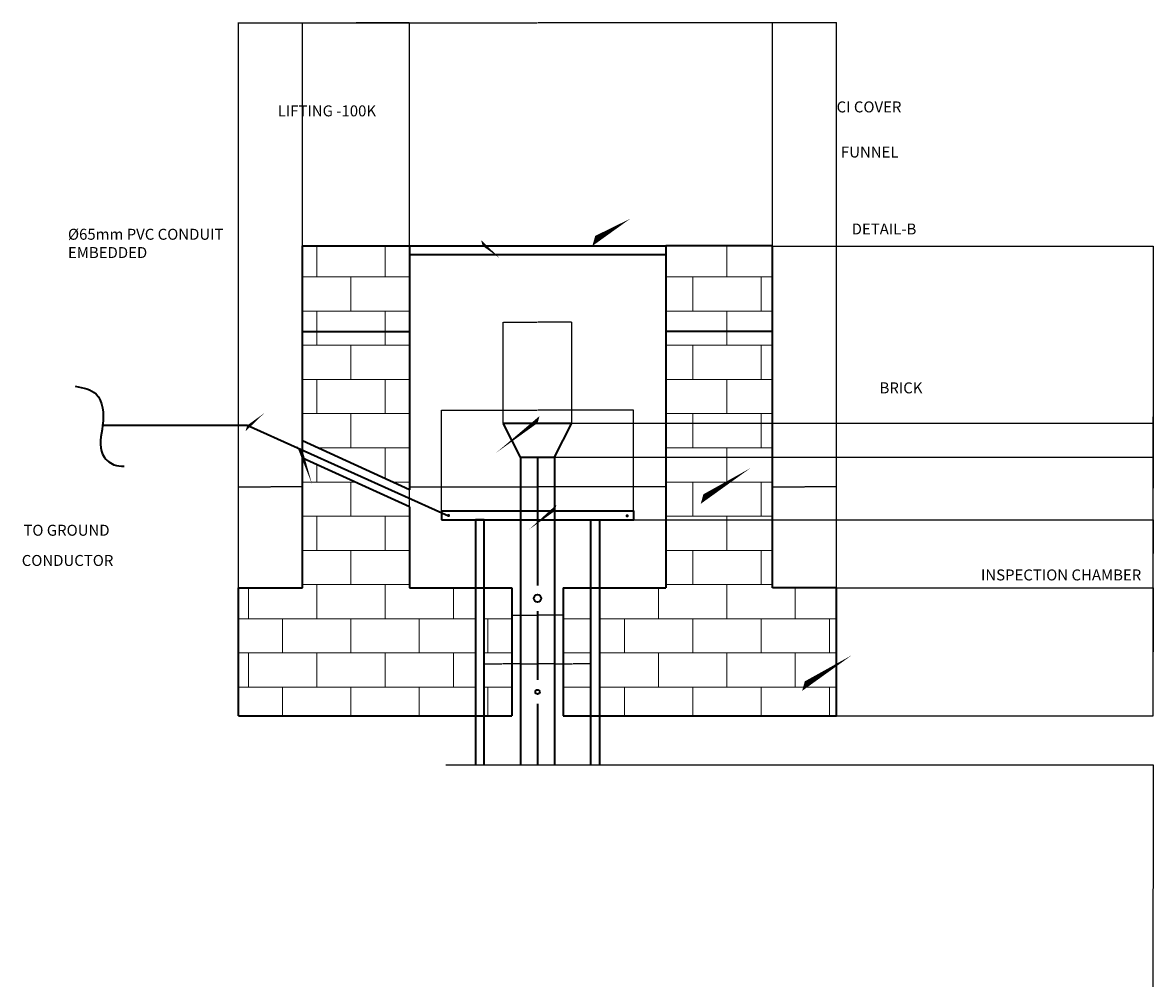
# Model space of a CAD drawing. Units: inches. Extents: x -514 to 1130, y -1450 to 978.
# Tile 2 of 2: x -224 to 1099, y -141 to 978. Entities that reach past the tile are written whole.
import ezdxf

# ---------------------------------------------------------------- set-up
doc = ezdxf.new("R2010")
doc.units = ezdxf.units.IN
doc.header["$MEASUREMENT"] = 0
for name, color, linetype, lineweight in [('A-ANNO-DIMS', 2, 'Continuous', 18), ('A-WALL', 7, 'Continuous', 35), ('A-WALL-PATT', 8, 'Continuous', 13), ('C-TOPO', 3, 'Continuous', 25), ('E-ANNO-LEAD', 2, 'Continuous', 18), ('E-ANNO-TEXT', 7, 'Continuous', 18), ('E-GRND', 1, 'Continuous', 35)]:
    doc.layers.add(name, color=color, linetype=linetype, lineweight=lineweight)
doc.styles.get("Standard").update_dxf_attribs({"font": 'arial.ttf'})
doc.dimstyles.get("Standard").update_dxf_attribs({"dimtxt": 0.18, "dimasz": 0.18, "dimexe": 0.18, "dimexo": 0.0625, "dimgap": 0.09, "dimtad": 0, "dimtih": 1, "dimtoh": 1, "dimdec": 4, "dimzin": 0, "dimdsep": 46, "dimtxsty": 'Standard', "dimcen": 0.09, "dimadec": 0, "dimazin": 0, "dimtfac": 1, "dimtdec": 4, "dimtofl": 0, "dimtmove": 0, "dimatfit": 3, "dimfxl": 1, "dimtolj": 1, "dimtzin": 0, "dimarcsym": 0})

# ---------------------------------------------------------------- blocks, each defined once
blk = doc.blocks.new('*D7')
at = {"layer": 'A-ANNO-DIMS', "color": 0, "lineweight": -2, "transparency": 16777216}
for p, q in [((103.4, 716.3), (103.4, 977.6)), ((103.6, 977.4), (378.1, 977.4)), ((653.2, 977.4), (378.7, 977.4)), ((653.4, 716.3), (653.4, 977.6))]:
    blk.add_line(p, q, dxfattribs=at)
at = {"layer": 'A-ANNO-DIMS', "color": 0, "transparency": 16777216}
for points in [[(103.6, 977.5), (103.6, 977.4), (103.4, 977.4)], [(653.2, 977.5), (653.2, 977.4), (653.4, 977.4)]]:
    blk.add_solid(points, dxfattribs=at)
at = {"layer": 'Defpoints', "color": 0, "transparency": 16777216}
for p in [(653.4, 977.4), (103.4, 716.2), (653.4, 716.2)]:
    blk.add_point(p, dxfattribs=at)
at = {"layer": 'A-ANNO-DIMS', "color": 0, "transparency": 16777216, "insert": (378.4, 977.4), "char_height": 0.18, "attachment_point": 5}
blk.add_mtext('\\A1;550', dxfattribs=at)
blk = doc.blocks.new('*D8')
at = {"layer": 'A-ANNO-DIMS', "color": 0, "lineweight": -2, "transparency": 16777216}
for p, q in [((103.4, 716.3), (103.4, 977.6)), ((103.6, 977.4), (165.6, 977.4)), ((228.2, 977.4), (166.2, 977.4)), ((228.4, 716.3), (228.4, 977.6))]:
    blk.add_line(p, q, dxfattribs=at)
at = {"layer": 'A-ANNO-DIMS', "color": 0, "transparency": 16777216}
for points in [[(103.6, 977.5), (103.6, 977.4), (103.4, 977.4)], [(228.2, 977.5), (228.2, 977.4), (228.4, 977.4)]]:
    blk.add_solid(points, dxfattribs=at)
at = {"layer": 'Defpoints', "color": 0, "transparency": 16777216}
for p in [(228.4, 977.4), (103.4, 716.2), (228.4, 716.2)]:
    blk.add_point(p, dxfattribs=at)
at = {"layer": 'A-ANNO-DIMS', "color": 0, "transparency": 16777216, "insert": (165.9, 977.4), "char_height": 0.18, "attachment_point": 5}
blk.add_mtext('\\A1;125', dxfattribs=at)
blk = doc.blocks.new('*D9')
at = {"layer": 'A-ANNO-DIMS', "color": 0, "lineweight": -2, "transparency": 16777216}
for p, q in [((228.4, 316.3), (228.4, 434.4)), ((228.6, 434.2), (378.1, 434.2)), ((528.2, 434.2), (378.7, 434.2)), ((528.4, 316.3), (528.4, 434.4))]:
    blk.add_line(p, q, dxfattribs=at)
at = {"layer": 'A-ANNO-DIMS', "color": 0, "transparency": 16777216}
for points in [[(228.6, 434.3), (228.6, 434.2), (228.4, 434.2)], [(528.2, 434.3), (528.2, 434.2), (528.4, 434.2)]]:
    blk.add_solid(points, dxfattribs=at)
at = {"layer": 'Defpoints', "color": 0, "transparency": 16777216}
for p in [(528.4, 434.2), (228.4, 316.2), (528.4, 316.2)]:
    blk.add_point(p, dxfattribs=at)
at = {"layer": 'A-ANNO-DIMS', "color": 0, "transparency": 16777216, "insert": (378.4, 434.2), "char_height": 0.18, "attachment_point": 5}
blk.add_mtext('\\A1;300', dxfattribs=at)
blk = doc.blocks.new('*D10')
at = {"layer": 'A-ANNO-DIMS', "color": 0, "lineweight": -2, "transparency": 16777216}
for p, q in [((28.4, 316.3), (28.4, 977.6)), ((28.6, 977.4), (378.1, 977.4)), ((728.2, 977.4), (378.7, 977.4)), ((728.4, 316.3), (728.4, 977.6))]:
    blk.add_line(p, q, dxfattribs=at)
at = {"layer": 'A-ANNO-DIMS', "color": 0, "transparency": 16777216}
for points in [[(28.6, 977.5), (28.6, 977.4), (28.4, 977.4)], [(728.2, 977.5), (728.2, 977.4), (728.4, 977.4)]]:
    blk.add_solid(points, dxfattribs=at)
at = {"layer": 'Defpoints', "color": 0, "transparency": 16777216}
for p in [(728.4, 977.4), (28.4, 316.2), (728.4, 316.2)]:
    blk.add_point(p, dxfattribs=at)
at = {"layer": 'A-ANNO-DIMS', "color": 0, "transparency": 16777216, "insert": (378.4, 977.4), "char_height": 0.18, "attachment_point": 5}
blk.add_mtext('\\A1;700', dxfattribs=at)
blk = doc.blocks.new('*D11')
at = {"layer": 'A-ANNO-DIMS', "color": 0, "lineweight": -2, "transparency": 16777216}
for p, q in [((28.4, 316.3), (28.4, 434.4)), ((28.6, 434.2), (65.7, 434.2)), ((103.2, 434.2), (66.1, 434.2)), ((103.4, 316.3), (103.4, 434.4))]:
    blk.add_line(p, q, dxfattribs=at)
at = {"layer": 'A-ANNO-DIMS', "color": 0, "transparency": 16777216}
for points in [[(28.6, 434.3), (28.6, 434.2), (28.4, 434.2)], [(103.2, 434.3), (103.2, 434.2), (103.4, 434.2)]]:
    blk.add_solid(points, dxfattribs=at)
at = {"layer": 'Defpoints', "color": 0, "transparency": 16777216}
for p in [(103.4, 434.2), (28.4, 316.2), (103.4, 316.2)]:
    blk.add_point(p, dxfattribs=at)
at = {"layer": 'A-ANNO-DIMS', "color": 0, "transparency": 16777216, "insert": (65.9, 434.2), "char_height": 0.18, "attachment_point": 5}
blk.add_mtext('\\A1;75', dxfattribs=at)
blk = doc.blocks.new('*D12')
at = {"layer": 'A-ANNO-DIMS', "color": 0, "lineweight": -2, "transparency": 16777216}
for p, q in [((653.4, 316.3), (653.4, 434.4)), ((653.6, 434.2), (690.7, 434.2)), ((728.2, 434.2), (691.1, 434.2)), ((728.4, 316.3), (728.4, 434.4))]:
    blk.add_line(p, q, dxfattribs=at)
at = {"layer": 'A-ANNO-DIMS', "color": 0, "transparency": 16777216}
for points in [[(653.6, 434.3), (653.6, 434.2), (653.4, 434.2)], [(728.2, 434.3), (728.2, 434.2), (728.4, 434.2)]]:
    blk.add_solid(points, dxfattribs=at)
at = {"layer": 'Defpoints', "color": 0, "transparency": 16777216}
for p in [(728.4, 434.2), (653.4, 316.2), (728.4, 316.2)]:
    blk.add_point(p, dxfattribs=at)
at = {"layer": 'A-ANNO-DIMS', "color": 0, "transparency": 16777216, "insert": (690.9, 434.2), "char_height": 0.18, "attachment_point": 5}
blk.add_mtext('\\A1;75', dxfattribs=at)
blk = doc.blocks.new('*D13')
at = {"layer": 'A-ANNO-DIMS', "color": 0, "lineweight": -2, "transparency": 16777216}
for p, q in [((348.4, 166.3), (348.4, 284.4)), ((348.6, 284.2), (378.2, 284.2)), ((408.2, 284.2), (378.6, 284.2)), ((408.4, 166.3), (408.4, 284.4))]:
    blk.add_line(p, q, dxfattribs=at)
at = {"layer": 'A-ANNO-DIMS', "color": 0, "transparency": 16777216}
for points in [[(348.6, 284.3), (348.6, 284.2), (348.4, 284.2)], [(408.2, 284.3), (408.2, 284.2), (408.4, 284.2)]]:
    blk.add_solid(points, dxfattribs=at)
at = {"layer": 'Defpoints', "color": 0, "transparency": 16777216}
for p in [(408.4, 284.2), (348.4, 166.2), (408.4, 166.2)]:
    blk.add_point(p, dxfattribs=at)
at = {"layer": 'A-ANNO-DIMS', "color": 0, "transparency": 16777216, "insert": (378.4, 284.2), "char_height": 0.18, "attachment_point": 5}
blk.add_mtext('\\A1;60', dxfattribs=at)
blk = doc.blocks.new('*D14')
at = {"layer": 'A-ANNO-DIMS', "color": 0, "lineweight": -2, "transparency": 16777216}
for p, q in [((653.5, 716.2), (1099, 716.2)), ((1098.9, 716.1), (1098.9, 516.4)), ((1098.9, 316.4), (1098.9, 516.1)), ((653.5, 316.2), (1099, 316.2))]:
    blk.add_line(p, q, dxfattribs=at)
at = {"layer": 'A-ANNO-DIMS', "color": 0, "transparency": 16777216}
for points in [[(1098.8, 716.1), (1098.9, 716.1), (1098.9, 716.2)], [(1098.8, 316.4), (1098.9, 316.4), (1098.9, 316.2)]]:
    blk.add_solid(points, dxfattribs=at)
at = {"layer": 'Defpoints', "color": 0, "transparency": 16777216}
for p in [(653.4, 716.2), (1098.9, 716.2), (653.4, 316.2)]:
    blk.add_point(p, dxfattribs=at)
at = {"layer": 'A-ANNO-DIMS', "color": 0, "transparency": 16777216, "insert": (1098.9, 516.2), "char_height": 0.18, "attachment_point": 5}
blk.add_mtext('\\A1;400', dxfattribs=at)
blk = doc.blocks.new('*D15')
at = {"layer": 'A-ANNO-DIMS', "color": 0, "lineweight": -2, "transparency": 16777216}
for p, q in [((728.5, 316.2), (1099, 316.2)), ((1098.9, 316.1), (1098.9, 241.4)), ((1098.9, 166.4), (1098.9, 241.1)), ((728.5, 166.2), (1099, 166.2))]:
    blk.add_line(p, q, dxfattribs=at)
at = {"layer": 'A-ANNO-DIMS', "color": 0, "transparency": 16777216}
for points in [[(1098.8, 316.1), (1098.9, 316.1), (1098.9, 316.2)], [(1098.8, 166.4), (1098.9, 166.4), (1098.9, 166.2)]]:
    blk.add_solid(points, dxfattribs=at)
at = {"layer": 'Defpoints', "color": 0, "transparency": 16777216}
for p in [(728.4, 316.2), (1098.9, 316.2), (728.4, 166.2)]:
    blk.add_point(p, dxfattribs=at)
at = {"layer": 'A-ANNO-DIMS', "color": 0, "transparency": 16777216, "insert": (1098.9, 241.2), "char_height": 0.18, "attachment_point": 5}
blk.add_mtext('\\A1;150', dxfattribs=at)
blk = doc.blocks.new('*D16')
at = {"layer": 'A-ANNO-DIMS', "color": 0, "lineweight": -2, "transparency": 16777216}
for p, q in [((653.5, 716.2), (1099, 716.2)), ((1098.9, 716.1), (1098.9, 441.4)), ((1098.9, 166.4), (1098.9, 441.1)), ((728.5, 166.2), (1099, 166.2))]:
    blk.add_line(p, q, dxfattribs=at)
at = {"layer": 'A-ANNO-DIMS', "color": 0, "transparency": 16777216}
for points in [[(1098.8, 716.1), (1098.9, 716.1), (1098.9, 716.2)], [(1098.8, 166.4), (1098.9, 166.4), (1098.9, 166.2)]]:
    blk.add_solid(points, dxfattribs=at)
at = {"layer": 'Defpoints', "color": 0, "transparency": 16777216}
for p in [(653.4, 716.2), (1098.9, 716.2), (728.4, 166.2)]:
    blk.add_point(p, dxfattribs=at)
at = {"layer": 'A-ANNO-DIMS', "color": 0, "transparency": 16777216, "insert": (1098.9, 441.2), "char_height": 0.18, "attachment_point": 5}
blk.add_mtext('\\A1;550', dxfattribs=at)
blk = doc.blocks.new('*D17')
at = {"layer": 'A-ANNO-DIMS', "color": 0, "lineweight": -2, "transparency": 16777216}
for p, q in [((338.3, 509.1), (338.3, 627.2)), ((338.5, 627), (378, 627)), ((418.3, 627), (378.8, 627)), ((418.5, 509.1), (418.5, 627.2))]:
    blk.add_line(p, q, dxfattribs=at)
at = {"layer": 'A-ANNO-DIMS', "color": 0, "transparency": 16777216}
for points in [[(338.5, 627), (338.5, 627), (338.3, 627)], [(418.3, 627), (418.3, 627), (418.5, 627)]]:
    blk.add_solid(points, dxfattribs=at)
at = {"layer": 'Defpoints', "color": 0, "transparency": 16777216}
for p in [(418.5, 627), (338.3, 509), (418.5, 509)]:
    blk.add_point(p, dxfattribs=at)
at = {"layer": 'A-ANNO-DIMS', "color": 0, "transparency": 16777216, "insert": (378.4, 627), "char_height": 0.18, "attachment_point": 5}
blk.add_mtext('\\A1;80.24', dxfattribs=at)
blk = doc.blocks.new('*D18')
at = {"layer": 'A-ANNO-DIMS', "color": 0, "lineweight": -2, "transparency": 16777216}
for p, q in [((265.9, 406), (265.9, 524.1)), ((266.1, 523.9), (378.1, 523.9)), ((490.7, 523.9), (378.7, 523.9)), ((490.9, 406), (490.9, 524.1))]:
    blk.add_line(p, q, dxfattribs=at)
at = {"layer": 'A-ANNO-DIMS', "color": 0, "transparency": 16777216}
for points in [[(266.1, 524), (266.1, 523.9), (265.9, 523.9)], [(490.7, 524), (490.7, 523.9), (490.9, 523.9)]]:
    blk.add_solid(points, dxfattribs=at)
at = {"layer": 'Defpoints', "color": 0, "transparency": 16777216}
for p in [(490.9, 523.9), (265.9, 405.9), (490.9, 405.9)]:
    blk.add_point(p, dxfattribs=at)
at = {"layer": 'A-ANNO-DIMS', "color": 0, "transparency": 16777216, "insert": (378.4, 523.9), "char_height": 0.18, "attachment_point": 5}
blk.add_mtext('\\A1;225', dxfattribs=at)
blk = doc.blocks.new('*D19')
at = {"layer": 'A-ANNO-DIMS', "color": 0, "lineweight": -2, "transparency": 16777216}
for p, q in [((491, 395.9), (1099, 395.9)), ((1098.9, 395.8), (1098.9, 356.3)), ((1098.9, 316.4), (1098.9, 355.9)), ((728.5, 316.2), (1099, 316.2))]:
    blk.add_line(p, q, dxfattribs=at)
at = {"layer": 'A-ANNO-DIMS', "color": 0, "transparency": 16777216}
for points in [[(1098.8, 395.8), (1098.9, 395.8), (1098.9, 395.9)], [(1098.8, 316.4), (1098.9, 316.4), (1098.9, 316.2)]]:
    blk.add_solid(points, dxfattribs=at)
at = {"layer": 'Defpoints', "color": 0, "transparency": 16777216}
for p in [(490.9, 395.9), (1098.9, 395.9), (728.4, 316.2)]:
    blk.add_point(p, dxfattribs=at)
at = {"layer": 'A-ANNO-DIMS', "color": 0, "transparency": 16777216, "insert": (1098.9, 356.1), "char_height": 0.18, "attachment_point": 5}
blk.add_mtext('\\A1;79.7', dxfattribs=at)
blk = doc.blocks.new('*D20')
at = {"layer": 'A-ANNO-DIMS', "color": 0, "lineweight": -2, "transparency": 16777216}
for p, q in [((398.5, 469), (1099, 469)), ((1098.9, 468.8), (1098.9, 432.7)), ((1098.9, 396.1), (1098.9, 432.3)), ((491, 395.9), (1099, 395.9))]:
    blk.add_line(p, q, dxfattribs=at)
at = {"layer": 'A-ANNO-DIMS', "color": 0, "transparency": 16777216}
for points in [[(1098.8, 468.8), (1098.9, 468.8), (1098.9, 469)], [(1098.8, 396.1), (1098.9, 396.1), (1098.9, 395.9)]]:
    blk.add_solid(points, dxfattribs=at)
at = {"layer": 'Defpoints', "color": 0, "transparency": 16777216}
for p in [(398.4, 469), (1098.9, 469), (490.9, 395.9)]:
    blk.add_point(p, dxfattribs=at)
at = {"layer": 'A-ANNO-DIMS', "color": 0, "transparency": 16777216, "insert": (1098.9, 432.5), "char_height": 0.18, "attachment_point": 5}
blk.add_mtext('\\A1;73.06', dxfattribs=at)
blk = doc.blocks.new('*D21')
at = {"layer": 'A-ANNO-DIMS', "color": 0, "lineweight": -2, "transparency": 16777216}
for p, q in [((418.6, 509), (1099, 509)), ((1098.9, 508.8), (1098.9, 489.2)), ((1098.9, 469.2), (1098.9, 488.8)), ((398.5, 469), (1099, 469))]:
    blk.add_line(p, q, dxfattribs=at)
at = {"layer": 'A-ANNO-DIMS', "color": 0, "transparency": 16777216}
for points in [[(1098.8, 508.8), (1098.9, 508.8), (1098.9, 509)], [(1098.8, 469.2), (1098.9, 469.2), (1098.9, 469)]]:
    blk.add_solid(points, dxfattribs=at)
at = {"layer": 'Defpoints', "color": 0, "transparency": 16777216}
for p in [(418.5, 509), (1098.9, 509), (398.4, 469)]:
    blk.add_point(p, dxfattribs=at)
at = {"layer": 'A-ANNO-DIMS', "color": 0, "transparency": 16777216, "insert": (1098.9, 489), "char_height": 0.18, "attachment_point": 5}
blk.add_mtext('\\A1;40', dxfattribs=at)
blk = doc.blocks.new('*D22')
at = {"layer": 'A-ANNO-DIMS', "color": 0, "lineweight": -2, "transparency": 16777216}
for p, q in [((491.3, 109.1), (1099, 109.1)), ((1098.9, 108.9), (1098.9, -35.7)), ((1098.9, -180.7), (1098.9, -36.1)), ((491.3, -180.9), (1099, -180.9))]:
    blk.add_line(p, q, dxfattribs=at)
at = {"layer": 'A-ANNO-DIMS', "color": 0, "transparency": 16777216}
for points in [[(1098.8, 108.9), (1098.9, 108.9), (1098.9, 109.1)], [(1098.8, -180.7), (1098.9, -180.7), (1098.9, -180.9)]]:
    blk.add_solid(points, dxfattribs=at)
at = {"layer": 'Defpoints', "color": 0, "transparency": 16777216}
for p in [(491.2, 109.1), (491.2, -180.9), (1098.9, -180.9)]:
    blk.add_point(p, dxfattribs=at)
at = {"layer": 'A-ANNO-DIMS', "color": 0, "transparency": 16777216, "insert": (1098.9, -35.9), "char_height": 0.18, "attachment_point": 5}
blk.add_mtext('\\A1;290', dxfattribs=at)
blk = doc.blocks.new('*D23')
at = {"layer": 'A-ANNO-DIMS', "color": 0, "lineweight": -2, "transparency": 16777216}
for p, q in [((315.9, 109.2), (315.9, 227.3)), ((316.1, 227.1), (336.8, 227.1)), ((358.2, 227.1), (337.5, 227.1)), ((358.4, 109.2), (358.4, 227.3))]:
    blk.add_line(p, q, dxfattribs=at)
at = {"layer": 'A-ANNO-DIMS', "color": 0, "transparency": 16777216}
for points in [[(316.1, 227.1), (316.1, 227.1), (315.9, 227.1)], [(358.2, 227.1), (358.2, 227.1), (358.4, 227.1)]]:
    blk.add_solid(points, dxfattribs=at)
at = {"layer": 'Defpoints', "color": 0, "transparency": 16777216}
for p in [(358.4, 227.1), (315.9, 109.1), (358.4, 109.1)]:
    blk.add_point(p, dxfattribs=at)
at = {"layer": 'A-ANNO-DIMS', "color": 0, "transparency": 16777216, "insert": (337.2, 227.1), "char_height": 0.18, "attachment_point": 5}
blk.add_mtext('\\A1;42.5', dxfattribs=at)
blk = doc.blocks.new('*D24')
at = {"layer": 'A-ANNO-DIMS', "color": 0, "lineweight": -2, "transparency": 16777216}
for p, q in [((358.4, 109.2), (358.4, 227.3)), ((358.6, 227.1), (378.2, 227.1)), ((398.2, 227.1), (378.6, 227.1)), ((398.4, 109.2), (398.4, 227.3))]:
    blk.add_line(p, q, dxfattribs=at)
at = {"layer": 'A-ANNO-DIMS', "color": 0, "transparency": 16777216}
for points in [[(358.6, 227.1), (358.6, 227.1), (358.4, 227.1)], [(398.2, 227.1), (398.2, 227.1), (398.4, 227.1)]]:
    blk.add_solid(points, dxfattribs=at)
at = {"layer": 'Defpoints', "color": 0, "transparency": 16777216}
for p in [(398.4, 227.1), (358.4, 109.1), (398.4, 109.1)]:
    blk.add_point(p, dxfattribs=at)
at = {"layer": 'A-ANNO-DIMS', "color": 0, "transparency": 16777216, "insert": (378.4, 227.1), "char_height": 0.18, "attachment_point": 5}
blk.add_mtext('\\A1;40', dxfattribs=at)
blk = doc.blocks.new('*D25')
at = {"layer": 'A-ANNO-DIMS', "color": 0, "lineweight": -2, "transparency": 16777216}
for p, q in [((398.4, 109.2), (398.4, 227.3)), ((398.6, 227.1), (419.3, 227.1)), ((440.7, 227.1), (420, 227.1)), ((440.9, 109.2), (440.9, 227.3))]:
    blk.add_line(p, q, dxfattribs=at)
at = {"layer": 'A-ANNO-DIMS', "color": 0, "transparency": 16777216}
for points in [[(398.6, 227.1), (398.6, 227.1), (398.4, 227.1)], [(440.7, 227.1), (440.7, 227.1), (440.9, 227.1)]]:
    blk.add_solid(points, dxfattribs=at)
at = {"layer": 'Defpoints', "color": 0, "transparency": 16777216}
for p in [(440.9, 227.1), (398.4, 109.1), (440.9, 109.1)]:
    blk.add_point(p, dxfattribs=at)
at = {"layer": 'A-ANNO-DIMS', "color": 0, "transparency": 16777216, "insert": (419.7, 227.1), "char_height": 0.18, "attachment_point": 5}
blk.add_mtext('\\A1;42.5', dxfattribs=at)

msp = doc.modelspace()

# ---------------------------------------------------------------- hatches: boundary and pattern name
at = {"layer": 'A-WALL-PATT'}
h = msp.add_hatch(dxfattribs=at)
h.set_pattern_fill('AR-B816', color=256, scale=5)
h.paths.add_polyline_path([(653.4114, 616.249), (528.4114, 616.249), (528.4114, 316.249), (450.9114, 316.249), (450.9114, 166.249), (728.4114, 166.249), (728.4114, 316.249), (653.4114, 316.249)])
h.paths.add_polyline_path([(305.9114, 316.249), (228.4114, 316.249), (228.4114, 410.9574), (103.4114, 468.1138), (103.4114, 316.249), (28.4114, 316.249), (28.4114, 166.249), (305.9114, 166.249)])
h.paths.add_polyline_path([(228.4114, 616.249), (103.4114, 616.249), (103.4114, 488.1138), (228.4114, 430.9574)])
h.paths.add_polyline_path([(228.4114, 716.249), (103.4114, 716.249), (103.4114, 616.249), (228.4114, 616.249)])
h.paths.add_polyline_path([(653.4114, 716.249), (528.4114, 716.249), (528.4114, 616.249), (653.4114, 616.249)])
h.paths.add_polyline_path([(440.9114, 316.249), (408.4114, 316.249), (408.4114, 166.249), (440.9114, 166.249)])
h.paths.add_polyline_path([(348.4114, 316.249), (315.9114, 316.249), (315.9114, 166.249), (348.4114, 166.249)])

# ---------------------------------------------------------------- linework, layer by layer
at = {"layer": 'A-WALL'}
for p, q in [((103.4114, 616.249), (103.4114, 716.249)), ((103.4114, 716.249), (228.4114, 716.249)), ((228.4114, 716.249), (228.4114, 430.9574)), ((228.4114, 716.249), (528.4114, 716.249)), ((653.4114, 716.249), (528.4114, 716.249)), ((528.4114, 716.249), (528.4114, 316.249)), ((653.4114, 616.249), (653.4114, 716.249)), ((228.4114, 706.249), (528.4114, 706.249)), ((103.4114, 316.249), (103.4114, 616.249)), ((103.4114, 616.249), (228.4114, 616.249)), ((653.4114, 616.249), (528.4114, 616.249)), ((653.4114, 316.249), (653.4114, 616.249)), ((228.4114, 410.9574), (228.4114, 316.249)), ((28.4114, 166.249), (28.4114, 316.249)), ((28.4114, 316.249), (103.4114, 316.249)), ((228.4114, 316.249), (348.4114, 316.249)), ((348.4114, 316.249), (348.4114, 166.249)), ((408.4114, 316.249), (408.4114, 166.249)), ((408.4114, 316.249), (528.4114, 316.249)), ((728.4114, 316.249), (653.4114, 316.249)), ((728.4114, 166.249), (728.4114, 316.249)), ((28.4114, 166.249), (348.4114, 166.249)), ((408.4114, 166.249), (728.4114, 166.249))]:
    msp.add_line(p, q, dxfattribs=at)
at = {"layer": 'C-TOPO'}
msp.add_line((270.9153, 109.1003), (491.2068, 109.1003), dxfattribs=at)
at = {"layer": 'E-ANNO-LEAD'}
for points in [[(314.2552, 716.249, 0, 13.2101, 0), (303.4419, 731.6936, 0, 0, 0), (176.2337, 854.7943, 0, 0, 0), (78.7042, 854.7943, 0, 0, 0)], [(442.5675, 716.249, 0, 13.2101, 0), (453.3808, 731.6936, 0, 0, 0), (713.8075, 859.4291, 0, 0, 0), (811.337, 859.4291, 0, 0, 0)], [(378.4114, 509.005, 0, 13.2101, 0), (389.2247, 524.4496, 0, 0, 0), (720.5228, 805.2712, 0, 0, 0), (818.0523, 805.2712, 0, 0, 0)], [(103.4114, 477.0187, 0, 13.2101, 0), (92.5981, 492.4634, 0, 0, 0), (5.3322, 711.6798, 0, 0, 0), (-92.1973, 711.6798, 0, 0, 0)], [(398.4114, 405.9479, 0, 13.2101, 0), (409.2247, 421.3926, 0, 0, 0), (733.0904, 715.2065, 0, 0, 0), (830.6199, 715.2065, 0, 0, 0)], [(569.3742, 414.4714, 0, 13.2101, 0), (580.1875, 429.9161, 0, 0, 0), (764.6621, 532.5402, 0, 0, 0), (862.1916, 532.5402, 0, 0, 0)], [(38.6026, 506.271, 0, 13.2101, 0), (27.7893, 490.8264, 0, 0, 0), (-99.419, 367.7257, 0, 0, 0), (-196.9485, 367.7257, 0, 0, 0)], [(688.0417, 195.5595, 0, 13.2101, 0), (698.8551, 211.0042, 0, 0, 0), (883.3297, 313.6283, 0, 0, 0), (980.8592, 313.6283, 0, 0, 0)]]:
    msp.add_lwpolyline(points, format="xyseb", dxfattribs=at)
at = {"layer": 'E-GRND'}
for p, q in [((338.2929, 509.005), (418.5299, 509.005)), ((358.4114, 469.005), (338.2929, 509.005)), ((398.4114, 469.005), (418.5299, 509.005)), ((228.4114, 430.9574), (103.4114, 488.1138)), ((228.4114, 410.9574), (103.4114, 468.1138)), ((358.4114, 469.005), (358.4114, 109.1003)), ((358.4114, 469.005), (398.4114, 469.005)), ((378.4114, 469.005), (378.4114, 318.8462)), ((398.4114, 469.005), (398.4114, 109.1003)), ((378.4114, 289.0527), (378.4114, 208.3643)), ((378.4114, 180.477), (378.4114, 109.1003))]:
    msp.add_line(p, q, dxfattribs=at)
for points in [[(274.1943, 399.9336), (38.6026, 506.271), (-130.6439, 506.271)], [(315.9114, 109.1003), (315.9114, 395.9479), (305.9114, 395.9479), (305.9114, 109.1003)], [(440.9114, 109.1003), (440.9114, 395.9479), (450.9114, 395.9479), (450.9114, 109.1003)]]:
    msp.add_lwpolyline(points, dxfattribs=at)
msp.add_lwpolyline([(265.9114, 395.9479), (490.9114, 395.9479), (490.9114, 405.9479), (265.9114, 405.9479)], close=True, dxfattribs=at)
at = {"layer": 'E-GRND', "const_width": 1.8371}
for points in [[(273.2757, 400.8522, 1), (275.1129, 400.8522, 1)], [(482.4261, 400.4516, 1), (484.2632, 400.4516, 1)]]:
    msp.add_lwpolyline(points, format="xyb", close=True, dxfattribs=at)
at = {"layer": 'E-GRND'}
for centre, radius in [((378.4114, 303.8804), 4.3406), ((378.4114, 194.3618), 2.5732)]:
    msp.add_circle(centre, radius, dxfattribs=at)
msp.add_open_spline([(-162.6127, 552.2927), (-153.2664, 550.3376), (-130.5747, 545.5911), (-128.2521, 506.4742), (-137.3734, 476.2741), (-119.6812, 459.0706), (-109.4357, 458.5737), (-105.257, 458.371)], degree=3, knots=[0, 0, 0, 0, 26.188829756, 63.58266363, 97.394470601, 115.34887117, 127.715725173, 127.715725173, 127.715725173, 127.715725173], dxfattribs=at)

# ---------------------------------------------------------------- texts
at = {"layer": 'E-ANNO-TEXT'}
for s, height, p in [('LIFTING -100K', 12.829888, (74.311, 867.9068)), ('CI COVER', 12.82989, (728.424, 872.5415)), ('FUNNEL', 12.82989, (733.4808, 819.7636)), ('DETAIL-B', 12.82989, (746.0484, 729.6989)), ('BRICK', 12.82989, (778.6886, 543.775)), ('TO GROUND', 12.82989, (-223.3294, 377.1509)), ('CONDUCTOR', 12.82989, (-225.2744, 341.7834)), ('INSPECTION CHAMBER', 12.829888, (897.3561, 324.863))]:
    msp.add_text(s, height=height, dxfattribs=at).set_placement(p)
at = {"layer": 'E-ANNO-TEXT', "insert": (-171.1715, 736.3474), "char_height": 12.829888, "width": 218.032909, "attachment_point": 1}
msp.add_mtext('%%C65mm PVC CONDUIT\\PEMBEDDED', dxfattribs=at)

# ---------------------------------------------------------------- dimensions: what is measured, and where the dimension line sits
at = {"layer": 'A-ANNO-DIMS'}
for base, p1, p2, override, picture, middle in [((728.4114, 977.4291), (28.4114, 316.249), (728.4114, 316.249), {"dimdec": 0, "dimlfac": 1, "dimrnd": 0, "dimzin": 0, "dimdsep": 46, "dimlunit": 2}, '*D10', (378.4114, 977.4291)), ((653.4114, 977.4291), (103.4114, 716.249), (653.4114, 716.249), {"dimdec": 0, "dimlfac": 1, "dimrnd": 0, "dimzin": 0, "dimdsep": 46, "dimlunit": 2}, '*D7', (378.4114, 977.4291)), ((228.4114, 977.4291), (103.4114, 716.249), (228.4114, 716.249), {"dimdec": 0, "dimlfac": 1, "dimrnd": 0, "dimzin": 0, "dimdsep": 46, "dimlunit": 2}, '*D8', (165.9114, 977.4291)), ((103.4114, 434.249), (28.4114, 316.249), (103.4114, 316.249), {"dimdec": 0, "dimlfac": 1, "dimrnd": 0, "dimzin": 0, "dimdsep": 46, "dimlunit": 2}, '*D11', (65.9114, 434.249)), ((528.4114, 434.249), (228.4114, 316.249), (528.4114, 316.249), {"dimdec": 0, "dimlfac": 1, "dimrnd": 0, "dimzin": 0, "dimdsep": 46, "dimlunit": 2}, '*D9', (378.4114, 434.249)), ((728.4114, 434.249), (653.4114, 316.249), (728.4114, 316.249), {"dimdec": 0, "dimlfac": 1, "dimrnd": 0, "dimzin": 0, "dimdsep": 46, "dimlunit": 2}, '*D12', (690.9114, 434.249)), ((408.4114, 284.249), (348.4114, 166.249), (408.4114, 166.249), {"dimdec": 0, "dimlfac": 1, "dimrnd": 0, "dimzin": 0, "dimdsep": 46, "dimlunit": 2}, '*D13', (378.4114, 284.249)), ((398.4114, 227.1003), (358.4114, 109.1003), (398.4114, 109.1003), {"dimdec": 0, "dimlfac": 1, "dimrnd": 0, "dimzin": 0, "dimdsep": 46, "dimlunit": 2}, '*D24', (378.4114, 227.1003)), ((440.9114, 227.1003), (398.4114, 109.1003), (440.9114, 109.1003), {"dimdec": 1, "dimlfac": 1, "dimrnd": 0, "dimzin": 0, "dimdsep": 46, "dimlunit": 2}, '*D25', (419.6614, 227.1003))]:
    dim = msp.add_linear_dim(base=base, p1=p1, p2=p2, dimstyle='Standard', override=override, dxfattribs=at)
    dim.commit()
    dim.dimension.update_dxf_attribs({"geometry": picture, "text_midpoint": middle})
for base, p1, p2, angle, override, picture, middle in [((1098.8592, 716.249), (653.4114, 316.249), (653.4114, 716.249), 90, {"dimdec": 0, "dimlfac": 1, "dimrnd": 0, "dimzin": 0, "dimdsep": 46, "dimlunit": 2}, '*D14', (1098.8592, 516.249)), ((1098.8592, 716.249), (728.4114, 166.249), (653.4114, 716.249), 90, {"dimdec": 0, "dimlfac": 1, "dimrnd": 0, "dimzin": 0, "dimdsep": 46, "dimlunit": 2}, '*D16', (1098.8592, 441.249)), ((418.5299, 627.005), (338.2929, 509.005), (418.5299, 509.005), 0, {"dimdec": 2, "dimlfac": 1, "dimrnd": 0, "dimzin": 0, "dimdsep": 46, "dimlunit": 2}, '*D17', (378.4114, 627.005)), ((490.9114, 523.9479), (265.9114, 405.9479), (490.9114, 405.9479), 0, {"dimdec": 0, "dimlfac": 1, "dimrnd": 0, "dimzin": 0, "dimdsep": 46, "dimlunit": 2}, '*D18', (378.4114, 523.9479)), ((1098.8592, 509.005), (398.4114, 469.005), (418.5299, 509.005), 90, {"dimdec": 0, "dimlfac": 1, "dimrnd": 0, "dimzin": 0, "dimdsep": 46, "dimlunit": 2}, '*D21', (1098.8592, 489.005)), ((1098.8592, 469.005), (490.9114, 395.9479), (398.4114, 469.005), 90, {"dimdec": 2, "dimlfac": 1, "dimrnd": 0, "dimzin": 0, "dimdsep": 46, "dimlunit": 2}, '*D20', (1098.8592, 432.4764)), ((1098.8592, 395.9479), (728.4114, 316.249), (490.9114, 395.9479), 90, {"dimdec": 1, "dimlfac": 1, "dimrnd": 0, "dimzin": 0, "dimdsep": 46, "dimlunit": 2}, '*D19', (1098.8592, 356.0984)), ((1098.8592, 316.249), (728.4114, 166.249), (728.4114, 316.249), 90, {"dimdec": 0, "dimlfac": 1, "dimrnd": 0, "dimzin": 0, "dimdsep": 46, "dimlunit": 2}, '*D15', (1098.8592, 241.249)), ((358.4114, 227.1003), (315.9114, 109.1003), (358.4114, 109.1003), 0, {"dimdec": 1, "dimlfac": 1, "dimrnd": 0, "dimzin": 0, "dimdsep": 46, "dimlunit": 2}, '*D23', (337.1614, 227.1003)), ((1098.8592, -180.8997), (491.2068, 109.1003), (491.2068, -180.8997), 90, {"dimdec": 0, "dimlfac": 1, "dimrnd": 0, "dimzin": 0, "dimdsep": 46, "dimlunit": 2}, '*D22', (1098.8592, -35.8997))]:
    dim = msp.add_linear_dim(base=base, p1=p1, p2=p2, angle=angle, dimstyle='Standard', override=override, dxfattribs=at)
    dim.commit()
    dim.dimension.update_dxf_attribs({"geometry": picture, "text_midpoint": middle})

doc.saveas('drawing.dxf')
